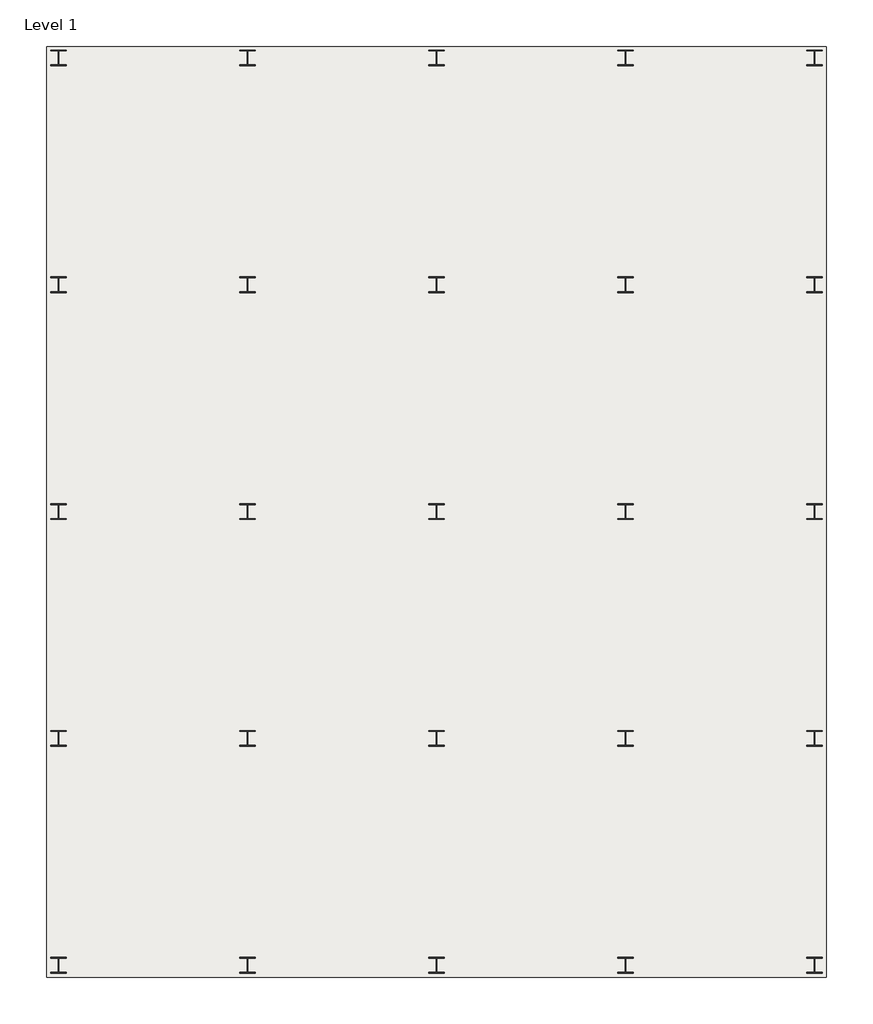
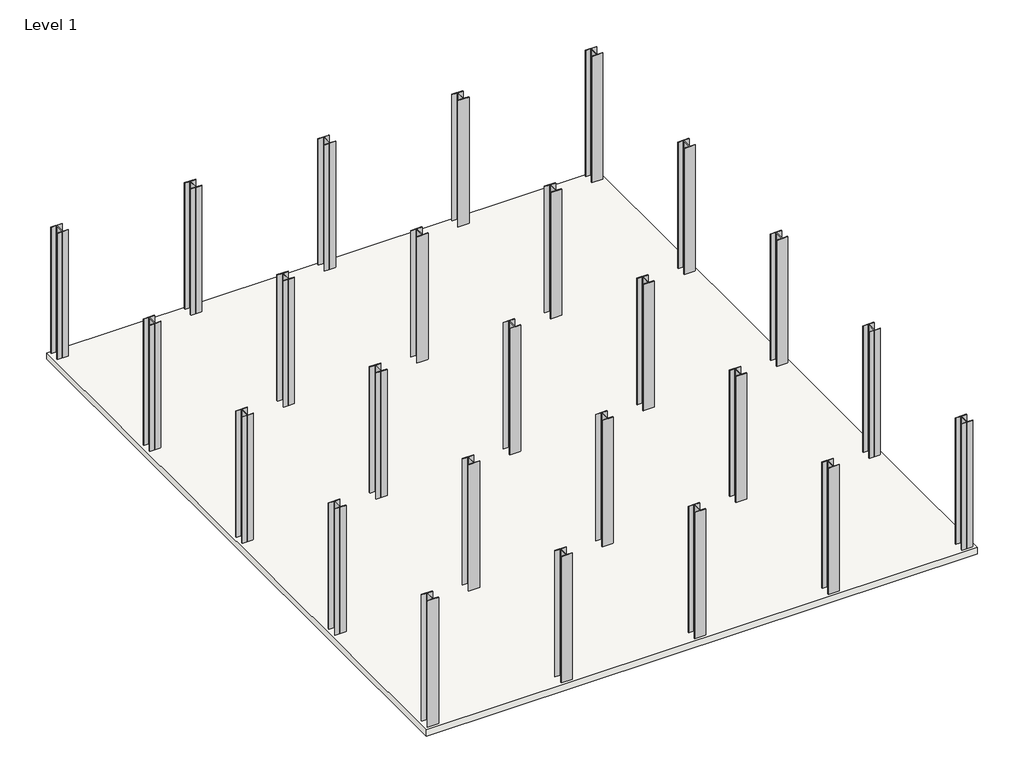
# One storey: 25 columns, 1 slab.
"""IFC4 building model written with IfcOpenShell, lengths in millimetres."""

from ifc_helpers import new_model, si_unit, frame, origin, place, context, project, spatial, polyline, outline, extrude, transform, mapped, element, save
from components import w_shapes_column_w10x49_a631470e

model = new_model("IFC4")

# Units and contexts
model_context = context("Model", 3, world=origin())
ifc_project = project(units=[si_unit("LENGTHUNIT", "METRE", prefix="MILLI")], contexts=[model_context])

# Site, building, storey
site = spatial("IfcSite", under=ifc_project)
building = spatial("IfcBuilding", under=site)
storey = spatial("IfcBuildingStorey", under=building, Name="Level 1", Elevation=0.0)

# Columns
placement = place(None, origin())
w_shapes_column_w10x49_shape = w_shapes_column_w10x49_a631470e(model_context)
element("IfcColumn", 1, ObjectType="W Shapes-Column : W10X49", at=placement, inside=storey, context=model_context, shape_type="MappedRepresentation", body=[
    mapped(w_shapes_column_w10x49_shape, transform((4784.4813402, -2213.7239423, 0.0), x_axis=(1.0, 0.0, 0.0), y_axis=(0.0, 1.0, 0.0), z_axis=(0.0, 0.0, 1.0))),
])
element("IfcColumn", 2, ObjectType="W Shapes-Column : W10X49", at=placement, inside=storey, context=model_context, shape_type="MappedRepresentation", body=[
    mapped(w_shapes_column_w10x49_shape, transform((1736.4813402, -2213.7239423, 0.0), x_axis=(1.0, 0.0, 0.0), y_axis=(0.0, 1.0, 0.0), z_axis=(0.0, 0.0, 1.0))),
])
element("IfcColumn", 3, ObjectType="W Shapes-Column : W10X49", at=placement, inside=storey, context=model_context, shape_type="MappedRepresentation", body=[
    mapped(w_shapes_column_w10x49_shape, transform((-1311.5186598, -2213.7239423, 0.0), x_axis=(1.0, 0.0, 0.0), y_axis=(0.0, 1.0, 0.0), z_axis=(0.0, 0.0, 1.0))),
])
element("IfcColumn", 4, ObjectType="W Shapes-Column : W10X49", at=placement, inside=storey, context=model_context, shape_type="MappedRepresentation", body=[
    mapped(w_shapes_column_w10x49_shape, transform((-4359.5186598, -2213.7239423, 0.0), x_axis=(1.0, 0.0, 0.0), y_axis=(0.0, 1.0, 0.0), z_axis=(0.0, 0.0, 1.0))),
])
element("IfcColumn", 5, ObjectType="W Shapes-Column : W10X49", at=placement, inside=storey, context=model_context, shape_type="MappedRepresentation", body=[
    mapped(w_shapes_column_w10x49_shape, transform((-7407.5186598, -2213.7239423, 0.0), x_axis=(1.0, 0.0, 0.0), y_axis=(0.0, 1.0, 0.0), z_axis=(0.0, 0.0, 1.0))),
])
element("IfcColumn", 6, ObjectType="W Shapes-Column : W10X49", at=placement, inside=storey, context=model_context, shape_type="MappedRepresentation", body=[
    mapped(w_shapes_column_w10x49_shape, transform((4784.4813402, 1443.8760577, 0.0), x_axis=(1.0, 0.0, 0.0), y_axis=(0.0, 1.0, 0.0), z_axis=(0.0, 0.0, 1.0))),
])
element("IfcColumn", 7, ObjectType="W Shapes-Column : W10X49", at=placement, inside=storey, context=model_context, shape_type="MappedRepresentation", body=[
    mapped(w_shapes_column_w10x49_shape, transform((4784.4813402, 5101.4760577, 0.0), x_axis=(1.0, 0.0, 0.0), y_axis=(0.0, 1.0, 0.0), z_axis=(0.0, 0.0, 1.0))),
])
element("IfcColumn", 8, ObjectType="W Shapes-Column : W10X49", at=placement, inside=storey, context=model_context, shape_type="MappedRepresentation", body=[
    mapped(w_shapes_column_w10x49_shape, transform((4784.4813402, 8759.0760577, 0.0), x_axis=(1.0, 0.0, 0.0), y_axis=(0.0, 1.0, 0.0), z_axis=(0.0, 0.0, 1.0))),
])
element("IfcColumn", 9, ObjectType="W Shapes-Column : W10X49", at=placement, inside=storey, context=model_context, shape_type="MappedRepresentation", body=[
    mapped(w_shapes_column_w10x49_shape, transform((4784.4813402, 12416.6760577, 0.0), x_axis=(1.0, 0.0, 0.0), y_axis=(0.0, 1.0, 0.0), z_axis=(0.0, 0.0, 1.0))),
])
element("IfcColumn", 10, ObjectType="W Shapes-Column : W10X49", at=placement, inside=storey, context=model_context, shape_type="MappedRepresentation", body=[
    mapped(w_shapes_column_w10x49_shape, transform((1736.4813402, 1443.8760577, 0.0), x_axis=(1.0, 0.0, 0.0), y_axis=(0.0, 1.0, 0.0), z_axis=(0.0, 0.0, 1.0))),
])
element("IfcColumn", 11, ObjectType="W Shapes-Column : W10X49", at=placement, inside=storey, context=model_context, shape_type="MappedRepresentation", body=[
    mapped(w_shapes_column_w10x49_shape, transform((-1311.5186598, 1443.8760577, 0.0), x_axis=(1.0, 0.0, 0.0), y_axis=(0.0, 1.0, 0.0), z_axis=(0.0, 0.0, 1.0))),
])
element("IfcColumn", 12, ObjectType="W Shapes-Column : W10X49", at=placement, inside=storey, context=model_context, shape_type="MappedRepresentation", body=[
    mapped(w_shapes_column_w10x49_shape, transform((-4359.5186598, 1443.8760577, 0.0), x_axis=(1.0, 0.0, 0.0), y_axis=(0.0, 1.0, 0.0), z_axis=(0.0, 0.0, 1.0))),
])
element("IfcColumn", 13, ObjectType="W Shapes-Column : W10X49", at=placement, inside=storey, context=model_context, shape_type="MappedRepresentation", body=[
    mapped(w_shapes_column_w10x49_shape, transform((-7407.5186598, 1443.8760577, 0.0), x_axis=(1.0, 0.0, 0.0), y_axis=(0.0, 1.0, 0.0), z_axis=(0.0, 0.0, 1.0))),
])
element("IfcColumn", 14, ObjectType="W Shapes-Column : W10X49", at=placement, inside=storey, context=model_context, shape_type="MappedRepresentation", body=[
    mapped(w_shapes_column_w10x49_shape, transform((1736.4813402, 5101.4760577, 0.0), x_axis=(1.0, 0.0, 0.0), y_axis=(0.0, 1.0, 0.0), z_axis=(0.0, 0.0, 1.0))),
])
element("IfcColumn", 15, ObjectType="W Shapes-Column : W10X49", at=placement, inside=storey, context=model_context, shape_type="MappedRepresentation", body=[
    mapped(w_shapes_column_w10x49_shape, transform((-1311.5186598, 5101.4760577, 0.0), x_axis=(1.0, 0.0, 0.0), y_axis=(0.0, 1.0, 0.0), z_axis=(0.0, 0.0, 1.0))),
])
element("IfcColumn", 16, ObjectType="W Shapes-Column : W10X49", at=placement, inside=storey, context=model_context, shape_type="MappedRepresentation", body=[
    mapped(w_shapes_column_w10x49_shape, transform((-4359.5186598, 5101.4760577, 0.0), x_axis=(1.0, 0.0, 0.0), y_axis=(0.0, 1.0, 0.0), z_axis=(0.0, 0.0, 1.0))),
])
element("IfcColumn", 17, ObjectType="W Shapes-Column : W10X49", at=placement, inside=storey, context=model_context, shape_type="MappedRepresentation", body=[
    mapped(w_shapes_column_w10x49_shape, transform((-7407.5186598, 5101.4760577, 0.0), x_axis=(1.0, 0.0, 0.0), y_axis=(0.0, 1.0, 0.0), z_axis=(0.0, 0.0, 1.0))),
])
element("IfcColumn", 18, ObjectType="W Shapes-Column : W10X49", at=placement, inside=storey, context=model_context, shape_type="MappedRepresentation", body=[
    mapped(w_shapes_column_w10x49_shape, transform((1736.4813402, 8759.0760577, 0.0), x_axis=(1.0, 0.0, 0.0), y_axis=(0.0, 1.0, 0.0), z_axis=(0.0, 0.0, 1.0))),
])
element("IfcColumn", 19, ObjectType="W Shapes-Column : W10X49", at=placement, inside=storey, context=model_context, shape_type="MappedRepresentation", body=[
    mapped(w_shapes_column_w10x49_shape, transform((-1311.5186598, 8759.0760577, 0.0), x_axis=(1.0, 0.0, 0.0), y_axis=(0.0, 1.0, 0.0), z_axis=(0.0, 0.0, 1.0))),
])
element("IfcColumn", 20, ObjectType="W Shapes-Column : W10X49", at=placement, inside=storey, context=model_context, shape_type="MappedRepresentation", body=[
    mapped(w_shapes_column_w10x49_shape, transform((-4359.5186598, 8759.0760577, 0.0), x_axis=(1.0, 0.0, 0.0), y_axis=(0.0, 1.0, 0.0), z_axis=(0.0, 0.0, 1.0))),
])
element("IfcColumn", 21, ObjectType="W Shapes-Column : W10X49", at=placement, inside=storey, context=model_context, shape_type="MappedRepresentation", body=[
    mapped(w_shapes_column_w10x49_shape, transform((-7407.5186598, 8759.0760577, 0.0), x_axis=(1.0, 0.0, 0.0), y_axis=(0.0, 1.0, 0.0), z_axis=(0.0, 0.0, 1.0))),
])
element("IfcColumn", 22, ObjectType="W Shapes-Column : W10X49", at=placement, inside=storey, context=model_context, shape_type="MappedRepresentation", body=[
    mapped(w_shapes_column_w10x49_shape, transform((1736.4813402, 12416.6760577, 0.0), x_axis=(1.0, 0.0, 0.0), y_axis=(0.0, 1.0, 0.0), z_axis=(0.0, 0.0, 1.0))),
])
element("IfcColumn", 23, ObjectType="W Shapes-Column : W10X49", at=placement, inside=storey, context=model_context, shape_type="MappedRepresentation", body=[
    mapped(w_shapes_column_w10x49_shape, transform((-1311.5186598, 12416.6760577, 0.0), x_axis=(1.0, 0.0, 0.0), y_axis=(0.0, 1.0, 0.0), z_axis=(0.0, 0.0, 1.0))),
])
element("IfcColumn", 24, ObjectType="W Shapes-Column : W10X49", at=placement, inside=storey, context=model_context, shape_type="MappedRepresentation", body=[
    mapped(w_shapes_column_w10x49_shape, transform((-4359.5186598, 12416.6760577, 0.0), x_axis=(1.0, 0.0, 0.0), y_axis=(0.0, 1.0, 0.0), z_axis=(0.0, 0.0, 1.0))),
])
element("IfcColumn", 25, ObjectType="W Shapes-Column : W10X49", at=placement, inside=storey, context=model_context, shape_type="MappedRepresentation", body=[
    mapped(w_shapes_column_w10x49_shape, transform((-7407.5186598, 12416.6760577, 0.0), x_axis=(1.0, 0.0, 0.0), y_axis=(0.0, 1.0, 0.0), z_axis=(0.0, 0.0, 1.0))),
])

# Slab
element("IfcSlab", 26, ObjectType="6\" Foundation Slab", at=placement, inside=storey, context=model_context, shape_type="SweptSolid", body=[
    extrude(outline(polyline([(4974.3230176, 12600.4819642), (4974.3230176, -2410.9180358), (-7598.6769824, -2410.9180358), (-7598.6769824, 12600.4819642), (4974.3230176, 12600.4819642)])), frame((0.0, 0.0, -152.4), z_axis=(0.0, 0.0, 1.0), x_axis=(1.0, 0.0, 0.0)), (0.0, 0.0, 1.0), 152.4),
])

save(model, "model.ifc")

# Revit data of these elements
# Grids (mm)
#   "1": line (10335.134, -2213.724) -> (-27131.771, -2213.724)
#   "2": line (4784.481, -8725.066) -> (4784.481, 21163.063)
#   "3": line (10335.134, 1443.876) -> (-27131.771, 1443.876)
#   "4": line (10335.134, 5101.476) -> (-27131.771, 5101.476)
#   "5": line (10335.134, 8759.076) -> (-27131.771, 8759.076)
#   "6": line (10335.134, 12416.676) -> (-27131.771, 12416.676)
#   "7": line (1736.481, -8725.066) -> (1736.481, 21163.063)
#   "8": line (-1311.519, -8725.066) -> (-1311.519, 21163.063)
#   "9": line (-4359.519, -8725.066) -> (-4359.519, 21163.063)
#   "10": line (-7407.519, -8725.066) -> (-7407.519, 21163.063)
# Type "W Shapes-Column : W10X49"
#   Section Name Key = "W10x49"
#   Assembly Code = "B10"
#   Width = 10.000"
#   Web Thickness = 0.340"
#   Web Fillet = 0.500"
#   Warping Constant = 2070.00 in⁶
#   Torsional Moment of Inertia = 1.39 in⁴
#   Section Area = 14.40 in²
#   Plastic Modulus weak axis = 28.30 in³
#   Plastic Modulus strong axis = 60.40 in³
#   Perimeter = 58.50 ft²/ft
#   Nominal Weight = 49.00 lbf/ft
#   Moment of Inertia weak axis = 93.40 in⁴
#   Moment of Inertia strong axis = 272.00 in⁴
#   Height = 10.000"
#   Flange Thickness = 0.560"
#   Elastic Modulus weak axis = 18.70 in³
#   Elastic Modulus strong axis = 54.60 in³
#   Centroid Vertical = 5.000"
#   Centroid Horizontal = 5.000"
#   Bolt Spacing = 0' - 5 1/2"
#   Structural Material [instance default] = Steel ASTM A992
#   Principal Axes Angle = 0
# Type "6\" Foundation Slab"
#   Layers, outside or top first: 0' - 6" "Concrete, Cast-in-Place gray" (function 1)
# Elements 1, 2, 3, 4, 5, 6, 7, 8, 9, 10, 11, 12, 13, 14, 15, 16, 17, 18, 19, 20, 21, 22, 23, 24, 25 (IfcColumn, "W Shapes-Column : W10X49")
#   Structural Material = Steel ASTM A992
#   Phase Created = New Construction
#   Materials on its faces: "Steel ASTM A992"
# Element 26 (IfcSlab, "6\" Foundation Slab")
#   Height Offset From Level = 0' - 0"
#   built-in parameter 1001954 = 1
#   Phase Created = New Construction
#   Materials on its faces: "Concrete, Cast-in-Place gray"
# Materials
#   "Steel ASTM A992": class "Metal", colour RGB 199 199 199, transparency 0, Description = "Structural steel 50ksi", Cost = 0
#   "Concrete, Cast-in-Place gray": class "Concrete", colour RGB 192 192 192, transparency 0, Description = "Cast-in-place concrete", Cost = 0
